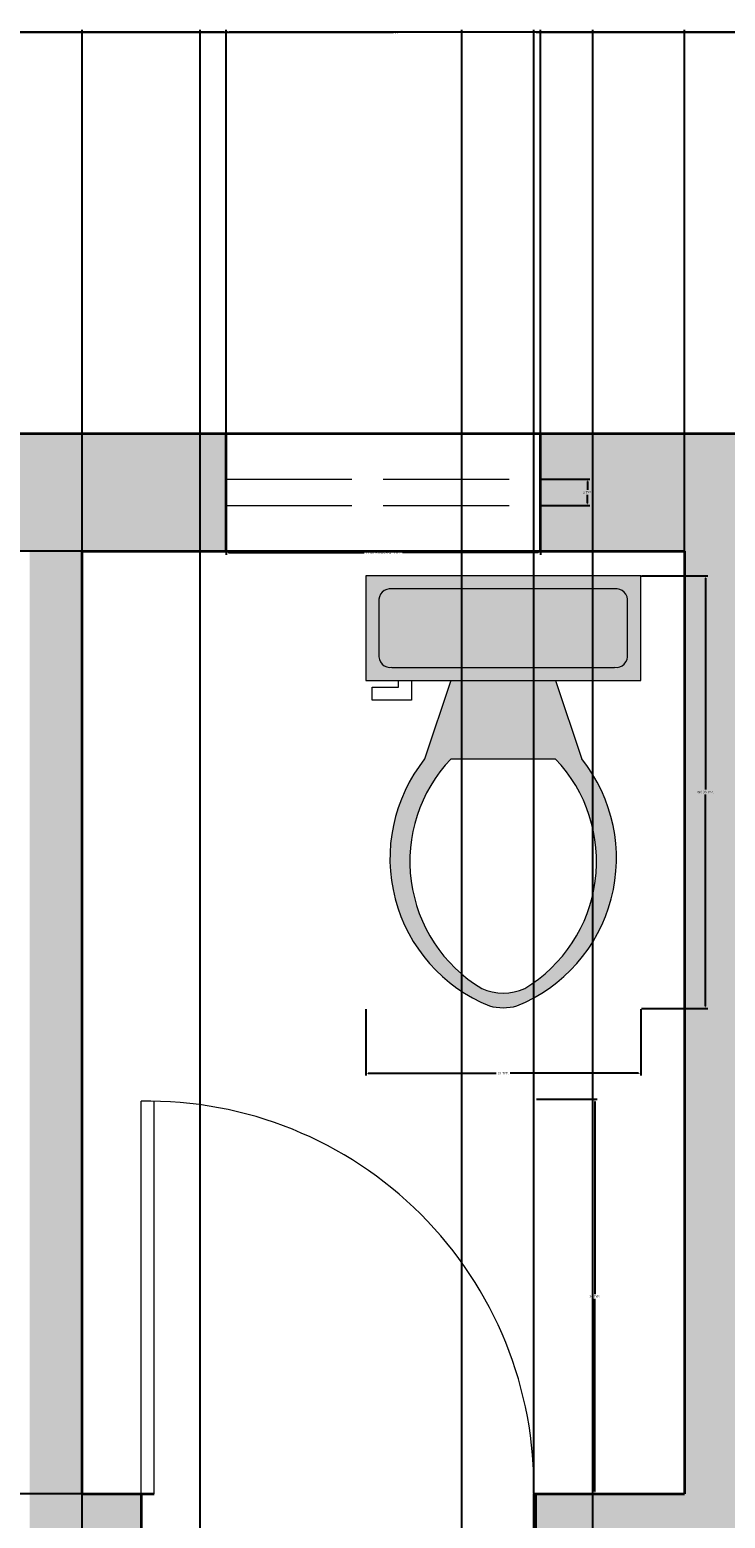
# Model space of a CAD drawing. Units: inches. Extents: x 1567 to 1964, y 1813 to 2447.
# Tile 26 of 28: x 1738 to 1792, y 2333 to 2447. Entities that reach past the tile are written whole.
import ezdxf

# ---------------------------------------------------------------- set-up
doc = ezdxf.new("R2010")
doc.units = ezdxf.units.IN
doc.linetypes.add('ACAD_ISO02W100', pattern=[15, 12, -3])
for name, color, linetype, lineweight in [('A-ANNO-DIMS', 2, 'Continuous', 18), ('A-DOOR', 4, 'Continuous', 18), ('A-FLOR-FIXT', 8, 'Continuous', 20), ('A-GLAZ-OVHD', 4, 'ACAD_ISO02W100', 18), ('A-WALL', 7, 'Continuous', 35)]:
    doc.layers.add(name, color=color, linetype=linetype, lineweight=lineweight)
doc.layers.add('A-FLOR-FIXT-PATT', color=252, linetype='Continuous', lineweight=13, true_color=0x939598)
doc.layers.add('A-WALL-PATT', color=251, linetype='Continuous', lineweight=13, true_color=0x636466)
doc.styles.get("Standard").update_dxf_attribs({"font": 'arial.ttf'})
doc.dimstyles.get("Standard").update_dxf_attribs({"dimtxt": 0.18, "dimasz": 0.18, "dimexe": 0.18, "dimexo": 0.0625, "dimgap": 0.09, "dimtad": 0, "dimtih": 1, "dimtoh": 1, "dimdec": 4, "dimzin": 0, "dimdsep": 46, "dimtxsty": 'Standard', "dimcen": 0.09, "dimadec": 0, "dimazin": 0, "dimtfac": 1, "dimtdec": 4, "dimtofl": 0, "dimtmove": 0, "dimatfit": 3, "dimfxl": 1, "dimtolj": 1, "dimtzin": 0, "dimarcsym": 0})

# ---------------------------------------------------------------- blocks, each defined once
blk = doc.blocks.new('Toilet - top')
for p, q in [((9.5, -6), (9.5, -2)), ((-10, -8.5), (-8, -8.5)), ((-10, -9.5), (-10, -8.5)), ((-8, -8.5), (-8, -8)), ((-7, -8), (-7, -9.5)), ((-4, -8), (-6, -14)), ((4, -8), (6, -14)), ((-7, -9.5), (-10, -9.5)), ((4, -14), (-4, -14))]:
    blk.add_line(p, q)
blk.add_lwpolyline([(10.5, -8), (10.5, 0), (-10.5, 0), (-10.5, -8)], close=True)
for points in [[(8.5, -1), (-8.5, -1)], [(-9.5, -2), (-9.5, -6)], [(-8.5, -7), (8.5, -7)]]:
    blk.add_lwpolyline(points)
for centre, radius, start, end in [((-8.62, -1.88), 0.884, 81.8699, 188.1301), ((8.62, -1.88), 0.884, 351.8699, 98.1301), ((-8.62, -6.12), 0.884, 171.8699, 278.1301), ((8.62, -6.12), 0.884, 261.8699, 8.1301), ((3.52, -21.58), 12.17, 141.4691, 247.9714), ((4.2, -21.82), 11.33, 136.3677, 238.9468), ((-3.52, -21.58), 12.17, 292.0284, 38.5307), ((-4.2, -21.82), 11.33, 301.053, 43.6321), ((0, -27.88), 4, 245.7318, 294.2682), ((0, -29), 4, 254.8605, 285.1395)]:
    blk.add_arc(centre, radius, start, end)
blk = doc.blocks.new('DOOR-SWING-30IN')
for p, q in [((0, 0), (0, 30)), ((1, 0), (1, 30))]:
    blk.add_line(p, q)
blk.add_arc((0.5, 0.5), 29.5, 359.029, 90.971)
blk = doc.blocks.new('WINDOW-24IN-HIGH')
at = {"ltscale": 0.8}
for p, q in [((0, 2), (24, 2)), ((0, 0), (24, 0))]:
    blk.add_line(p, q, dxfattribs=at)
blk = doc.blocks.new('*D19')
at = {"layer": 'A-ANNO-DIMS', "color": 0, "lineweight": -2, "transparency": 16777216}
for p, q in [((1785.15, 2405.42), (1790.22, 2405.42)), ((1790.04, 2405.24), (1790.04, 2389.08)), ((1790.04, 2372.55), (1790.04, 2388.71)), ((1785.15, 2372.37), (1790.22, 2372.37))]:
    blk.add_line(p, q, dxfattribs=at)
at = {"layer": 'A-ANNO-DIMS', "color": 0, "transparency": 16777216}
for points in [[(1790.01, 2405.24), (1790.07, 2405.24), (1790.04, 2405.42)], [(1790.01, 2372.55), (1790.07, 2372.55), (1790.04, 2372.37)]]:
    blk.add_solid(points, dxfattribs=at)
at = {"layer": 'Defpoints', "color": 0, "transparency": 16777216}
for p in [(1785.09, 2405.42), (1790.04, 2405.42), (1785.09, 2372.37)]:
    blk.add_point(p, dxfattribs=at)
at = {"layer": 'A-ANNO-DIMS', "color": 0, "transparency": 16777216, "insert": (1790.04, 2388.9), "char_height": 0.18, "attachment_point": 5}
blk.add_mtext('\\A1;WC 33 TYP.', dxfattribs=at)
blk = doc.blocks.new('*D20')
at = {"layer": 'A-ANNO-DIMS', "color": 0, "lineweight": -2, "transparency": 16777216}
for p, q in [((1764.09, 2372.31), (1764.09, 2367.24)), ((1785.09, 2372.31), (1785.09, 2367.24)), ((1764.27, 2367.42), (1774.06, 2367.42)), ((1784.91, 2367.42), (1775.11, 2367.42))]:
    blk.add_line(p, q, dxfattribs=at)
at = {"layer": 'A-ANNO-DIMS', "color": 0, "transparency": 16777216}
for points in [[(1764.27, 2367.45), (1764.27, 2367.39), (1764.09, 2367.42)], [(1784.91, 2367.45), (1784.91, 2367.39), (1785.09, 2367.42)]]:
    blk.add_solid(points, dxfattribs=at)
at = {"layer": 'Defpoints', "color": 0, "transparency": 16777216}
for p in [(1764.09, 2372.37), (1785.09, 2372.37), (1785.09, 2367.42)]:
    blk.add_point(p, dxfattribs=at)
at = {"layer": 'A-ANNO-DIMS', "color": 0, "transparency": 16777216, "insert": (1774.59, 2367.42), "char_height": 0.18, "attachment_point": 5}
blk.add_mtext('\\A1;21 TYP.', dxfattribs=at)
blk = doc.blocks.new('*D31')
at = {"layer": 'A-ANNO-DIMS', "color": 0, "lineweight": -2, "transparency": 16777216}
for p, q in [((1746.93, 2335.23), (1746.93, 2330.59)), ((1777.07, 2335.23), (1777.07, 2330.59)), ((1747.11, 2330.77), (1761.06, 2330.77)), ((1776.89, 2330.77), (1762.93, 2330.77))]:
    blk.add_line(p, q, dxfattribs=at)
at = {"layer": 'A-ANNO-DIMS', "color": 0, "transparency": 16777216}
for points in [[(1747.11, 2330.8), (1747.11, 2330.74), (1746.93, 2330.77)], [(1776.89, 2330.8), (1776.89, 2330.74), (1777.07, 2330.77)]]:
    blk.add_solid(points, dxfattribs=at)
at = {"layer": 'Defpoints', "color": 0, "transparency": 16777216}
for p in [(1746.93, 2335.29), (1777.07, 2335.29), (1777.07, 2330.77)]:
    blk.add_point(p, dxfattribs=at)
at = {"layer": 'A-ANNO-DIMS', "color": 0, "transparency": 16777216, "insert": (1762, 2330.77), "char_height": 0.18, "attachment_point": 5}
blk.add_mtext('\\A1;DOOR 30 TYP.', dxfattribs=at)
blk = doc.blocks.new('*D32')
at = {"layer": 'A-ANNO-DIMS', "color": 0, "lineweight": -2, "transparency": 16777216}
for p, q in [((1777.13, 2365.43), (1781.77, 2365.43)), ((1781.59, 2365.25), (1781.59, 2350.54)), ((1781.59, 2335.47), (1781.59, 2350.18)), ((1777.13, 2335.29), (1781.77, 2335.29))]:
    blk.add_line(p, q, dxfattribs=at)
at = {"layer": 'A-ANNO-DIMS', "color": 0, "transparency": 16777216}
for points in [[(1781.56, 2365.25), (1781.62, 2365.25), (1781.59, 2365.43)], [(1781.56, 2335.47), (1781.62, 2335.47), (1781.59, 2335.29)]]:
    blk.add_solid(points, dxfattribs=at)
at = {"layer": 'Defpoints', "color": 0, "transparency": 16777216}
for p in [(1777.07, 2365.43), (1781.59, 2365.43), (1777.07, 2335.29)]:
    blk.add_point(p, dxfattribs=at)
at = {"layer": 'A-ANNO-DIMS', "color": 0, "transparency": 16777216, "insert": (1781.59, 2350.36), "char_height": 0.18, "attachment_point": 5}
blk.add_mtext('\\A1;30 TYP.', dxfattribs=at)
blk = doc.blocks.new('*D37')
at = {"layer": 'A-ANNO-DIMS', "color": 0, "lineweight": -2, "transparency": 16777216}
for p, q in [((1753.43, 2410.73), (1753.43, 2407.01)), ((1777.43, 2410.73), (1777.43, 2407.01)), ((1753.61, 2407.19), (1763.97, 2407.19)), ((1777.25, 2407.19), (1766.89, 2407.19))]:
    blk.add_line(p, q, dxfattribs=at)
at = {"layer": 'A-ANNO-DIMS', "color": 0, "transparency": 16777216}
for points in [[(1753.61, 2407.22), (1753.61, 2407.16), (1753.43, 2407.19)], [(1777.25, 2407.22), (1777.25, 2407.16), (1777.43, 2407.19)]]:
    blk.add_solid(points, dxfattribs=at)
at = {"layer": 'Defpoints', "color": 0, "transparency": 16777216}
for p in [(1753.43, 2410.79), (1777.43, 2410.79), (1777.43, 2407.19)]:
    blk.add_point(p, dxfattribs=at)
at = {"layer": 'A-ANNO-DIMS', "color": 0, "transparency": 16777216, "insert": (1765.43, 2407.19), "char_height": 0.18, "attachment_point": 5}
blk.add_mtext('\\A1;HIGH WINDOW 24 TYP.', dxfattribs=at)
blk = doc.blocks.new('*D38')
at = {"layer": 'A-ANNO-DIMS', "color": 0, "lineweight": -2, "transparency": 16777216}
for p, q in [((1777.49, 2412.79), (1781.21, 2412.79)), ((1781.03, 2412.61), (1781.03, 2411.97)), ((1781.03, 2410.97), (1781.03, 2411.61)), ((1777.49, 2410.79), (1781.21, 2410.79))]:
    blk.add_line(p, q, dxfattribs=at)
at = {"layer": 'A-ANNO-DIMS', "color": 0, "transparency": 16777216}
for points in [[(1781, 2412.61), (1781.06, 2412.61), (1781.03, 2412.79)], [(1781, 2410.97), (1781.06, 2410.97), (1781.03, 2410.79)]]:
    blk.add_solid(points, dxfattribs=at)
at = {"layer": 'Defpoints', "color": 0, "transparency": 16777216}
for p in [(1777.43, 2412.79), (1781.03, 2412.79), (1777.43, 2410.79)]:
    blk.add_point(p, dxfattribs=at)
at = {"layer": 'A-ANNO-DIMS', "color": 0, "transparency": 16777216, "insert": (1781.03, 2411.79), "char_height": 0.18, "attachment_point": 5}
blk.add_mtext('\\A1;2 TYP.', dxfattribs=at)
blk = doc.blocks.new('*D44')
at = {"layer": 'A-ANNO-DIMS', "color": 0, "lineweight": -2, "transparency": 16777216}
for p, q in [((1690.43, 2416.35), (1690.43, 2447.12)), ((1690.61, 2446.94), (1721.71, 2446.94)), ((1753.25, 2446.94), (1722.15, 2446.94)), ((1753.43, 2416.35), (1753.43, 2447.12))]:
    blk.add_line(p, q, dxfattribs=at)
at = {"layer": 'A-ANNO-DIMS', "color": 0, "transparency": 16777216}
for points in [[(1690.61, 2446.97), (1690.61, 2446.91), (1690.43, 2446.94)], [(1753.25, 2446.97), (1753.25, 2446.91), (1753.43, 2446.94)]]:
    blk.add_solid(points, dxfattribs=at)
at = {"layer": 'Defpoints', "color": 0, "transparency": 16777216}
for p in [(1753.43, 2446.94), (1690.43, 2416.29), (1753.43, 2416.29)]:
    blk.add_point(p, dxfattribs=at)
at = {"layer": 'A-ANNO-DIMS', "color": 0, "transparency": 16777216, "insert": (1721.93, 2446.94), "char_height": 0.18, "attachment_point": 5}
blk.add_mtext('\\A1;63', dxfattribs=at)
blk = doc.blocks.new('*D45')
at = {"layer": 'A-ANNO-DIMS', "color": 0, "lineweight": -2, "transparency": 16777216}
for p, q in [((1777.43, 2416.35), (1777.43, 2447.12)), ((1777.61, 2446.94), (1808.71, 2446.94)), ((1840.25, 2446.94), (1809.15, 2446.94)), ((1840.43, 2416.35), (1840.43, 2447.12))]:
    blk.add_line(p, q, dxfattribs=at)
at = {"layer": 'A-ANNO-DIMS', "color": 0, "transparency": 16777216}
for points in [[(1777.61, 2446.97), (1777.61, 2446.91), (1777.43, 2446.94)], [(1840.25, 2446.97), (1840.25, 2446.91), (1840.43, 2446.94)]]:
    blk.add_solid(points, dxfattribs=at)
at = {"layer": 'Defpoints', "color": 0, "transparency": 16777216}
for p in [(1840.43, 2446.94), (1777.43, 2416.29), (1840.43, 2416.29)]:
    blk.add_point(p, dxfattribs=at)
at = {"layer": 'A-ANNO-DIMS', "color": 0, "transparency": 16777216, "insert": (1808.93, 2446.94), "char_height": 0.18, "attachment_point": 5}
blk.add_mtext('\\A1;63', dxfattribs=at)
blk = doc.blocks.new('*D48')
at = {"layer": 'A-ANNO-DIMS', "color": 0, "lineweight": -2, "transparency": 16777216}
for p, q in [((1742.37, 2407.29), (1566.6, 2407.29)), ((1566.78, 2407.11), (1566.78, 2371.47)), ((1566.78, 2335.47), (1566.78, 2371.11)), ((1742.37, 2335.29), (1566.6, 2335.29))]:
    blk.add_line(p, q, dxfattribs=at)
at = {"layer": 'A-ANNO-DIMS', "color": 0, "transparency": 16777216}
for points in [[(1566.75, 2407.11), (1566.81, 2407.11), (1566.78, 2407.29)], [(1566.75, 2335.47), (1566.81, 2335.47), (1566.78, 2335.29)]]:
    blk.add_solid(points, dxfattribs=at)
at = {"layer": 'Defpoints', "color": 0, "transparency": 16777216}
for p in [(1742.43, 2407.29), (1566.78, 2335.29), (1742.43, 2335.29)]:
    blk.add_point(p, dxfattribs=at)
at = {"layer": 'A-ANNO-DIMS', "color": 0, "transparency": 16777216, "insert": (1566.78, 2371.29), "char_height": 0.18, "attachment_point": 5}
blk.add_mtext('\\A1;72', dxfattribs=at)
blk = doc.blocks.new('*D49')
at = {"layer": 'A-ANNO-DIMS', "color": 0, "lineweight": -2, "transparency": 16777216}
for p, q in [((1776.93, 2335.35), (1776.93, 2447.12)), ((1777.11, 2446.94), (1782.36, 2446.94)), ((1788.25, 2446.94), (1783, 2446.94)), ((1788.43, 2335.35), (1788.43, 2447.12))]:
    blk.add_line(p, q, dxfattribs=at)
at = {"layer": 'A-ANNO-DIMS', "color": 0, "transparency": 16777216}
for points in [[(1777.11, 2446.97), (1777.11, 2446.91), (1776.93, 2446.94)], [(1788.25, 2446.97), (1788.25, 2446.91), (1788.43, 2446.94)]]:
    blk.add_solid(points, dxfattribs=at)
at = {"layer": 'Defpoints', "color": 0, "transparency": 16777216}
for p in [(1776.93, 2446.94), (1776.93, 2335.29), (1788.43, 2335.29)]:
    blk.add_point(p, dxfattribs=at)
at = {"layer": 'A-ANNO-DIMS', "color": 0, "transparency": 16777216, "insert": (1782.68, 2446.94), "char_height": 0.18, "attachment_point": 5}
blk.add_mtext('\\A1;11.5', dxfattribs=at)
blk = doc.blocks.new('*D54')
at = {"layer": 'A-ANNO-DIMS', "color": 0, "lineweight": -2, "transparency": 16777216}
for p, q in [((1711.43, 1964.35), (1711.43, 2447.12)), ((1711.61, 2446.94), (1753.21, 2446.94)), ((1795.25, 2446.94), (1753.65, 2446.94)), ((1795.43, 1964.35), (1795.43, 2447.12))]:
    blk.add_line(p, q, dxfattribs=at)
at = {"layer": 'A-ANNO-DIMS', "color": 0, "transparency": 16777216}
for points in [[(1711.61, 2446.97), (1711.61, 2446.91), (1711.43, 2446.94)], [(1795.25, 2446.97), (1795.25, 2446.91), (1795.43, 2446.94)]]:
    blk.add_solid(points, dxfattribs=at)
at = {"layer": 'Defpoints', "color": 0, "transparency": 16777216}
for p in [(1795.43, 2446.94), (1711.43, 1964.29), (1795.43, 1964.29)]:
    blk.add_point(p, dxfattribs=at)
at = {"layer": 'A-ANNO-DIMS', "color": 0, "transparency": 16777216, "insert": (1753.43, 2446.94), "char_height": 0.18, "attachment_point": 5}
blk.add_mtext('\\A1;84', dxfattribs=at)
blk = doc.blocks.new('*D58')
at = {"layer": 'A-ANNO-DIMS', "color": 0, "lineweight": -2, "transparency": 16777216}
for p, q in [((1742.43, 2127.35), (1742.43, 2447.12)), ((1742.61, 2446.94), (1746.78, 2446.94)), ((1751.25, 2446.94), (1747.08, 2446.94)), ((1751.43, 2127.35), (1751.43, 2447.12))]:
    blk.add_line(p, q, dxfattribs=at)
at = {"layer": 'A-ANNO-DIMS', "color": 0, "transparency": 16777216}
for points in [[(1742.61, 2446.97), (1742.61, 2446.91), (1742.43, 2446.94)], [(1751.25, 2446.97), (1751.25, 2446.91), (1751.43, 2446.94)]]:
    blk.add_solid(points, dxfattribs=at)
at = {"layer": 'Defpoints', "color": 0, "transparency": 16777216}
for p in [(1751.43, 2446.94), (1742.43, 2127.29), (1751.43, 2127.29)]:
    blk.add_point(p, dxfattribs=at)
at = {"layer": 'A-ANNO-DIMS', "color": 0, "transparency": 16777216, "insert": (1746.93, 2446.94), "char_height": 0.18, "attachment_point": 5}
blk.add_mtext('\\A1;9', dxfattribs=at)
blk = doc.blocks.new('*D59')
at = {"layer": 'A-ANNO-DIMS', "color": 0, "lineweight": -2, "transparency": 16777216}
for p, q in [((1751.43, 2127.35), (1751.43, 2447.12)), ((1751.61, 2446.94), (1766.21, 2446.94)), ((1781.25, 2446.94), (1766.65, 2446.94)), ((1781.43, 2127.35), (1781.43, 2447.12))]:
    blk.add_line(p, q, dxfattribs=at)
at = {"layer": 'A-ANNO-DIMS', "color": 0, "transparency": 16777216}
for points in [[(1751.61, 2446.97), (1751.61, 2446.91), (1751.43, 2446.94)], [(1781.25, 2446.97), (1781.25, 2446.91), (1781.43, 2446.94)]]:
    blk.add_solid(points, dxfattribs=at)
at = {"layer": 'Defpoints', "color": 0, "transparency": 16777216}
for p in [(1781.43, 2446.94), (1751.43, 2127.29), (1781.43, 2127.29)]:
    blk.add_point(p, dxfattribs=at)
at = {"layer": 'A-ANNO-DIMS', "color": 0, "transparency": 16777216, "insert": (1766.43, 2446.94), "char_height": 0.18, "attachment_point": 5}
blk.add_mtext('\\A1;30', dxfattribs=at)
blk = doc.blocks.new('*D63')
at = {"layer": 'A-ANNO-DIMS', "color": 0, "lineweight": -2, "transparency": 16777216}
for p, q in [((1735.43, 1988.35), (1735.43, 2447.12)), ((1735.61, 2446.94), (1753.21, 2446.94)), ((1771.25, 2446.94), (1753.65, 2446.94)), ((1771.43, 1988.35), (1771.43, 2447.12))]:
    blk.add_line(p, q, dxfattribs=at)
at = {"layer": 'A-ANNO-DIMS', "color": 0, "transparency": 16777216}
for points in [[(1735.61, 2446.97), (1735.61, 2446.91), (1735.43, 2446.94)], [(1771.25, 2446.97), (1771.25, 2446.91), (1771.43, 2446.94)]]:
    blk.add_solid(points, dxfattribs=at)
at = {"layer": 'Defpoints', "color": 0, "transparency": 16777216}
for p in [(1771.43, 2446.94), (1735.43, 1988.29), (1771.43, 1988.29)]:
    blk.add_point(p, dxfattribs=at)
at = {"layer": 'A-ANNO-DIMS', "color": 0, "transparency": 16777216, "insert": (1753.43, 2446.94), "char_height": 0.18, "attachment_point": 5}
blk.add_mtext('\\A1;36', dxfattribs=at)

msp = doc.modelspace()

# ---------------------------------------------------------------- hatches: boundary and pattern name
at = {"layer": 'A-FLOR-FIXT-PATT'}
h = msp.add_hatch(color=256, dxfattribs=at)
h.dxf.hatch_style = 1
h.paths.add_polyline_path([(1785.0853, 2405.4205), (1764.0853, 2405.4205), (1764.0853, 2397.4205), (1785.0853, 2397.4205)])
h.paths.add_polyline_path([(1783.0853, 2404.4205, -0.50000012), (1784.0853, 2403.4205), (1784.0853, 2399.4205, -0.50000012), (1783.0853, 2398.4205), (1766.0853, 2398.4205, -0.50000012), (1765.0853, 2399.4205), (1765.0853, 2403.4205, -0.50000012), (1766.0853, 2404.4205)], flags=0)
h.paths.add_polyline_path([(1784.0853, 2403.4205, 0.50000012), (1783.0853, 2404.4205), (1766.0853, 2404.4205, 0.50000012), (1765.0853, 2403.4205), (1765.0853, 2399.4205, 0.50000012), (1766.0853, 2398.4205), (1783.0853, 2398.4205, 0.50000012), (1784.0853, 2399.4205)], flags=16)
h.paths.add_polyline_path([(1784.0853, 2403.6705, 0.41421356), (1783.0853, 2404.4205), (1765.8353, 2404.4205, 0.41421356), (1765.0853, 2403.4205), (1765.0853, 2399.1705, 0.41421356), (1766.0853, 2398.4205), (1783.3353, 2398.4205, 0.41421356), (1784.0853, 2399.4205)], flags=0)
h = msp.add_hatch(color=256, dxfattribs=at)
h.dxf.hatch_style = 1
h.paths.add_polyline_path([(1785.0853, 2405.4205), (1764.0853, 2405.4205), (1764.0853, 2397.4205), (1785.0853, 2397.4205)])
h.paths.add_polyline_path([(1766.0853, 2404.4205, 0.50000012), (1765.0853, 2403.4205), (1765.0853, 2399.4205, 0.50000012), (1766.0853, 2398.4205), (1783.0853, 2398.4205, 0.50000012), (1784.0853, 2399.4205), (1784.0853, 2403.4205, 0.50000012), (1783.0853, 2404.4205)], flags=0)
h.paths.add_polyline_path([(1778.5853, 2397.4205), (1770.5853, 2397.4205), (1768.5853, 2391.4204, 0.50131678), (1773.5406, 2372.5594, 0.13289091), (1775.63, 2372.5594, 0.50132349), (1780.5853, 2391.4206)])
h.paths.add_polyline_path([(1778.5853, 2391.4205, -0.4800795), (1776.2293, 2373.8975, -0.21500378), (1772.9413, 2373.8975, -0.48007965), (1770.5853, 2391.4205)], flags=16)
h.paths.add_polyline_path([(1784.0853, 2403.6705, 0.41421356), (1783.0853, 2404.4205), (1765.8353, 2404.4205, 0.41421356), (1765.0853, 2403.4205), (1765.0853, 2399.1705, 0.41421356), (1766.0853, 2398.4205), (1783.3353, 2398.4205, 0.41421356), (1784.0853, 2399.4205)], flags=16)
h = msp.add_hatch(color=256, dxfattribs=at)
h.dxf.hatch_style = 1
h.paths.add_polyline_path([(1784.0853, 2403.6705, 0.41421356), (1783.0853, 2404.4205), (1765.8353, 2404.4205, 0.41421356), (1765.0853, 2403.4205), (1765.0853, 2399.1705, 0.41421356), (1766.0853, 2398.4205), (1783.3353, 2398.4205, 0.41421356), (1784.0853, 2399.4205)])
at = {"layer": 'A-WALL-PATT'}
h = msp.add_hatch(color=256, dxfattribs=at)
h.dxf.hatch_style = 1
h.paths.add_polyline_path([(1606.4295, 2407.29), (1654.4295, 2407.29), (1654.4295, 2416.29), (1597.4295, 2416.29), (1597.4295, 2217.29), (1606.4295, 2217.29), (1606.4295, 2259.29), (1738.4295, 2259.29), (1738.4295, 2247.29), (1742.4295, 2247.29), (1742.4295, 2259.29), (1742.4295, 2272.29), (1738.4295, 2272.29), (1738.4295, 2263.29), (1606.4295, 2263.29)])
h.paths.add_polyline_path([(1753.4295, 2416.29), (1690.4295, 2416.29), (1690.4295, 2407.29), (1738.4295, 2407.29), (1738.4295, 2308.29), (1742.4295, 2308.29), (1742.4295, 2331.29), (1746.9295, 2331.29), (1746.9295, 2335.29), (1742.4295, 2335.29), (1742.4295, 2407.29), (1753.4295, 2407.29)])
h.paths.add_polyline_path([(1840.4295, 2416.29), (1777.4295, 2416.29), (1777.4295, 2407.29), (1788.4295, 2407.29), (1788.4295, 2335.29), (1776.9295, 2335.29), (1776.9295, 2331.29), (1788.4295, 2331.29), (1788.4295, 2308.29), (1792.4295, 2308.29), (1792.4295, 2407.29), (1840.4295, 2407.29)])
h.paths.add_polyline_path([(1933.4295, 2416.29), (1876.4295, 2416.29), (1876.4295, 2407.29), (1924.4295, 2407.29), (1924.4295, 2263.29), (1792.4295, 2263.29), (1792.4295, 2272.29), (1788.4295, 2272.29), (1788.4295, 2259.29), (1872.4295, 2259.29), (1872.4295, 2171.29), (1880.9295, 2171.29), (1880.9295, 2175.29), (1876.4295, 2175.29), (1876.4295, 2259.29), (1924.4295, 2259.29), (1924.4295, 2229.29), (1933.4295, 2229.29)])
h.paths.add_polyline_path([(1933.4295, 2205.29), (1924.4295, 2205.29), (1924.4295, 2175.29), (1910.9295, 2175.29), (1910.9295, 2171.29), (1924.4295, 2171.29), (1924.4295, 2127.29), (1844.4295, 2127.29), (1844.4295, 2123.29), (1924.4295, 2123.29), (1924.4295, 2063.29), (1933.4295, 2063.29)])
h.paths.add_polyline_path([(1799.4295, 2123.29), (1808.4295, 2123.29), (1808.4295, 2127.29), (1781.4295, 2127.29), (1781.4295, 2123.29), (1795.4295, 2123.29), (1795.4295, 1964.29), (1711.4295, 1964.29), (1711.4295, 2123.29), (1751.4295, 2123.29), (1751.4295, 2127.29), (1742.4295, 2127.29), (1742.4295, 2139.29), (1738.4295, 2139.29), (1738.4295, 2127.29), (1678.4295, 2127.29), (1678.4295, 2123.29), (1702.4295, 2123.29), (1702.4295, 1913.29), (1678.4295, 1913.29), (1678.4295, 1904.29), (1711.4295, 1904.29), (1711.4295, 1960.29), (1795.4295, 1960.29), (1795.4295, 1906.69), (1929.4295, 1906.69), (1929.4295, 1848.29), (1601.4295, 1848.29), (1601.4295, 1904.29), (1630.4295, 1904.29), (1630.4295, 1913.29), (1606.4295, 1913.29), (1606.4295, 2123.29), (1630.4295, 2123.29), (1630.4295, 2127.29), (1606.4295, 2127.29), (1606.4295, 2169.29), (1597.4295, 2169.29), (1597.4295, 1844.29), (1933.4295, 1844.29), (1933.4295, 2027.29), (1924.4295, 2027.29), (1924.4295, 1967.29), (1833.9295, 1967.29), (1833.9295, 1963.29), (1924.4295, 1963.29), (1924.4295, 1910.69), (1799.4295, 1910.69), (1799.4295, 1963.29), (1803.9295, 1963.29), (1803.9295, 1967.29), (1799.4295, 1967.29)])

# ---------------------------------------------------------------- linework, layer by layer
at = {"layer": 'A-WALL'}
for p, q in [((1597.4295, 2416.29), (1933.4295, 2416.29)), ((1753.4295, 2407.29), (1753.4295, 2416.29)), ((1777.4295, 2407.29), (1777.4295, 2416.29)), ((1742.4295, 2407.29), (1788.4295, 2407.29)), ((1742.4295, 2335.29), (1742.4295, 2407.29)), ((1788.4295, 2407.29), (1788.4295, 2335.29)), ((1742.4295, 2335.29), (1747.9295, 2335.29)), ((1746.9295, 2335.29), (1746.9295, 2331.29)), ((1776.9295, 2335.29), (1776.9295, 2331.29)), ((1776.9295, 2335.29), (1788.4295, 2335.29))]:
    msp.add_line(p, q, dxfattribs=at)

# ---------------------------------------------------------------- block references
at = {"layer": 'A-DOOR'}
msp.add_blockref('DOOR-SWING-30IN', (1746.93, 2335.29), dxfattribs=at)
at = {"layer": 'A-FLOR-FIXT'}
msp.add_blockref('Toilet - top', (1774.5853, 2405.4205), dxfattribs=at)
at = {"layer": 'A-GLAZ-OVHD'}
msp.add_blockref('WINDOW-24IN-HIGH', (1753.43, 2410.79), dxfattribs=at)

# ---------------------------------------------------------------- dimensions: what is measured, and where the dimension line sits
at = {"layer": 'A-ANNO-DIMS'}
for base, p1, p2, override, picture, middle in [((1753.4295, 2446.94), (1690.4295, 2416.29), (1753.4295, 2416.29), {"dimdec": 0, "dimlfac": 1, "dimrnd": 0, "dimzin": 0, "dimdsep": 46, "dimlunit": 2}, '*D44', (1721.9295, 2446.94)), ((1795.4295, 2446.94), (1711.4295, 1964.29), (1795.4295, 1964.29), {"dimdec": 0, "dimlfac": 1, "dimrnd": 0, "dimzin": 0, "dimdsep": 46, "dimlunit": 2}, '*D54', (1753.4295, 2446.94)), ((1771.4295, 2446.94), (1735.4295, 1988.29), (1771.4295, 1988.29), {"dimdec": 0, "dimlfac": 1, "dimrnd": 0, "dimzin": 0, "dimdsep": 46, "dimlunit": 2}, '*D63', (1753.4295, 2446.94)), ((1751.4295, 2446.94), (1742.4295, 2127.29), (1751.4295, 2127.29), {"dimdec": 0, "dimlfac": 1, "dimrnd": 0, "dimzin": 0, "dimdsep": 46, "dimlunit": 2}, '*D58', (1746.9295, 2446.94)), ((1781.4295, 2446.94), (1751.4295, 2127.29), (1781.4295, 2127.29), {"dimdec": 0, "dimlfac": 1, "dimrnd": 0, "dimzin": 0, "dimdsep": 46, "dimlunit": 2}, '*D59', (1766.4295, 2446.94)), ((1776.9295, 2446.94), (1788.4295, 2335.29), (1776.9295, 2335.29), {"dimdec": 1, "dimlfac": 1, "dimrnd": 0, "dimzin": 0, "dimdsep": 46, "dimlunit": 2}, '*D49', (1782.6795, 2446.94)), ((1840.4295, 2446.94), (1777.4295, 2416.29), (1840.4295, 2416.29), {"dimdec": 0, "dimlfac": 1, "dimrnd": 0, "dimzin": 0, "dimdsep": 46, "dimlunit": 2}, '*D45', (1808.9295, 2446.94))]:
    dim = msp.add_linear_dim(base=base, p1=p1, p2=p2, dimstyle='Standard', override=override, dxfattribs=at)
    dim.commit()
    dim.dimension.update_dxf_attribs({"geometry": picture, "text_midpoint": middle})
for base, p1, p2, text, picture, middle in [((1781.0295, 2412.79), (1777.4295, 2410.79), (1777.4295, 2412.79), '<> TYP.', '*D38', (1781.0295, 2411.79)), ((1790.0422, 2405.4205), (1785.0853, 2372.3743), (1785.0853, 2405.4205), 'WC <> TYP.', '*D19', (1790.0422, 2388.8974)), ((1781.5854, 2365.4255), (1777.0651, 2335.29), (1777.0651, 2365.4255), '<> TYP.', '*D32', (1781.5854, 2350.3578))]:
    dim = msp.add_linear_dim(base=base, p1=p1, p2=p2, angle=90, text=text, dimstyle='Standard', override={"dimdec": 0, "dimlfac": 1, "dimrnd": 0, "dimzin": 0, "dimdsep": 46, "dimlunit": 2}, dxfattribs=at)
    dim.commit()
    dim.dimension.update_dxf_attribs({"geometry": picture, "text_midpoint": middle})
for base, p1, p2, text, picture, middle in [((1777.4295, 2407.19), (1753.4295, 2410.79), (1777.4295, 2410.79), 'HIGH WINDOW <> TYP.', '*D37', (1765.4295, 2407.19)), ((1785.0853, 2367.4173), (1764.0853, 2372.3743), (1785.0853, 2372.3743), '<> TYP.', '*D20', (1774.5853, 2367.4173)), ((1777.0651, 2330.7697), (1746.9295, 2335.29), (1777.0651, 2335.29), 'DOOR <> TYP.', '*D31', (1761.9973, 2330.7697))]:
    dim = msp.add_linear_dim(base=base, p1=p1, p2=p2, text=text, dimstyle='Standard', override={"dimdec": 0, "dimlfac": 1, "dimrnd": 0, "dimzin": 0, "dimdsep": 46, "dimlunit": 2}, dxfattribs=at)
    dim.commit()
    dim.dimension.update_dxf_attribs({"geometry": picture, "text_midpoint": middle})
dim = msp.add_linear_dim(base=(1566.7795, 2335.29), p1=(1742.4295, 2407.29), p2=(1742.4295, 2335.29), angle=90, dimstyle='Standard', override={"dimdec": 0, "dimlfac": 1, "dimrnd": 0, "dimzin": 0, "dimdsep": 46, "dimlunit": 2}, dxfattribs=at)
dim.commit()
dim.dimension.update_dxf_attribs({"geometry": '*D48', "text_midpoint": (1566.7795, 2371.29)})

doc.saveas('drawing.dxf')
